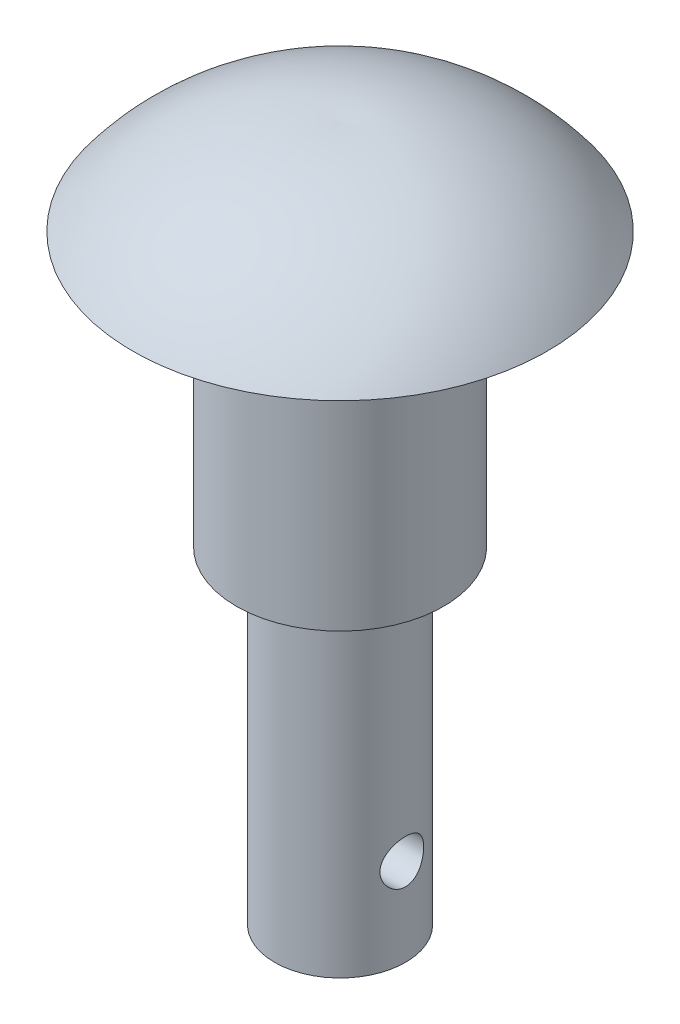
ISO-10303-21;
HEADER;
FILE_DESCRIPTION(('STEP AP214'),'2;1');
FILE_NAME('part.step','',(''),(''),'','','');
FILE_SCHEMA(('AUTOMOTIVE_DESIGN { 1 0 10303 214 1 1 1 1 }'));
ENDSEC;
DATA;
#1=APPLICATION_CONTEXT('core data for automotive mechanical design processes');
#2=APPLICATION_PROTOCOL_DEFINITION('international standard','automotive_design',2000,#1);
#3=PRODUCT_CONTEXT('',#1,'mechanical');
#4=PRODUCT('Part','Part','',(#3));
#5=PRODUCT_RELATED_PRODUCT_CATEGORY('part','',(#4));
#6=PRODUCT_DEFINITION_FORMATION('','',#4);
#7=PRODUCT_DEFINITION_CONTEXT('part definition',#1,'design');
#8=PRODUCT_DEFINITION('design','',#6,#7);
#9=PRODUCT_DEFINITION_SHAPE('','',#8);
#10=(LENGTH_UNIT() NAMED_UNIT(*) SI_UNIT(.MILLI.,.METRE.));
#11=(NAMED_UNIT(*) PLANE_ANGLE_UNIT() SI_UNIT($,.RADIAN.));
#12=(NAMED_UNIT(*) SI_UNIT($,.STERADIAN.) SOLID_ANGLE_UNIT());
#13=UNCERTAINTY_MEASURE_WITH_UNIT(LENGTH_MEASURE(1.E-05),#10,'distance_accuracy_value','');
#14=(GEOMETRIC_REPRESENTATION_CONTEXT(3) GLOBAL_UNCERTAINTY_ASSIGNED_CONTEXT((#13)) GLOBAL_UNIT_ASSIGNED_CONTEXT((#10,
#11,#12)) REPRESENTATION_CONTEXT('',''));
#15=CARTESIAN_POINT('',(0.,0.,0.));
#16=DIRECTION('',(0.,0.,1.));
#17=DIRECTION('',(1.,0.,0.));
#18=AXIS2_PLACEMENT_3D('',#15,#16,#17);
#19=CARTESIAN_POINT('',(0.,30.,0.));
#20=DIRECTION('',(0.,-1.,0.));
#21=DIRECTION('',(0.,0.,-1.));
#22=AXIS2_PLACEMENT_3D('',#19,#20,#21);
#23=CYLINDRICAL_SURFACE('',#22,6.);
#24=CARTESIAN_POINT('',(-5.65685424949238,8.,-2.));
#25=CARTESIAN_POINT('',(-5.65685389060868,8.10893634967214,-2.00000051589543));
#26=CARTESIAN_POINT('',(-5.66003538581715,8.21786959964719,-1.99106956737105));
#27=CARTESIAN_POINT('',(-5.67235148162509,8.4325088419885,-1.95570226337762));
#28=CARTESIAN_POINT('',(-5.68148706284377,8.53821429974494,-1.92926302433679));
#29=CARTESIAN_POINT('',(-5.70456407377583,8.74325378599457,-1.85991097136981));
#30=CARTESIAN_POINT('',(-5.71849607942643,8.84259985888543,-1.81703044280649));
#31=CARTESIAN_POINT('',(-5.74958244020649,9.03272009709592,-1.71612325688276));
#32=CARTESIAN_POINT('',(-5.76673750607224,9.12349236510726,-1.65809325772037));
#33=CARTESIAN_POINT('',(-5.80308978814946,9.29743992467663,-1.52610229288576));
#34=CARTESIAN_POINT('',(-5.82233789689288,9.38023085734346,-1.45164868275584));
#35=CARTESIAN_POINT('',(-5.86027729602006,9.53241360244928,-1.28997533442879));
#36=CARTESIAN_POINT('',(-5.87896849657923,9.60180326316474,-1.20275355010475));
#37=CARTESIAN_POINT('',(-5.91427733843598,9.72695779465919,-1.01520901593002));
#38=CARTESIAN_POINT('',(-5.93082815403211,9.78231994123592,-0.914603822449051));
#39=CARTESIAN_POINT('',(-5.95939173541966,9.87518317025502,-0.704862445974949));
#40=CARTESIAN_POINT('',(-5.97140572406004,9.91268906635381,-0.595728571374426));
#41=CARTESIAN_POINT('',(-5.98918150863813,9.96747170926479,-0.376057634866991));
#42=CARTESIAN_POINT('',(-5.99514629555118,9.98540689251401,-0.265701509705939));
#43=CARTESIAN_POINT('',(-6.00087216436495,10.0026325867213,-0.0433957496481808));
#44=CARTESIAN_POINT('',(-6.00063484525791,10.0019279033048,0.068553467087791));
#45=CARTESIAN_POINT('',(-5.99412079237462,9.98231149086794,0.286207030387628));
#46=CARTESIAN_POINT('',(-5.98808129510235,9.96411494305102,0.391984097183312));
#47=CARTESIAN_POINT('',(-5.97093934679463,9.91121403803906,0.598886877644342));
#48=CARTESIAN_POINT('',(-5.95983655262363,9.87650856204035,0.70001227555843));
#49=CARTESIAN_POINT('',(-5.93351340586448,9.79115736538788,0.896304949683944));
#50=CARTESIAN_POINT('',(-5.91824085048031,9.74030812290698,0.991376441937689));
#51=CARTESIAN_POINT('',(-5.88516786077838,9.62428058910269,1.17184865105464));
#52=CARTESIAN_POINT('',(-5.86736672402933,9.55909831334474,1.25724666877068));
#53=CARTESIAN_POINT('',(-5.83012383699793,9.4126512130806,1.42020173310261));
#54=CARTESIAN_POINT('',(-5.81064430337755,9.33077368431704,1.49720031413054));
#55=CARTESIAN_POINT('',(-5.77294670497801,9.15510254854676,1.63655451919635));
#56=CARTESIAN_POINT('',(-5.75472883491231,9.06130710854391,1.69890788656309));
#57=CARTESIAN_POINT('',(-5.72141050242224,8.86269274879312,1.80797491007149));
#58=CARTESIAN_POINT('',(-5.70635818569496,8.75773573736445,1.85445292724268));
#59=CARTESIAN_POINT('',(-5.68163301648769,8.54085721157116,1.92888638653867));
#60=CARTESIAN_POINT('',(-5.67195790974185,8.42893863758751,1.95684959149499));
#61=CARTESIAN_POINT('',(-5.6595927263117,8.20672328917685,1.99232256419504));
#62=CARTESIAN_POINT('',(-5.65660720637512,8.09658115050269,2.00069819101527));
#63=CARTESIAN_POINT('',(-5.65713344118368,7.87644770177179,1.99921087781944));
#64=CARTESIAN_POINT('',(-5.66064401583629,7.76645636795203,1.98935125045353));
#65=CARTESIAN_POINT('',(-5.67347236180599,7.55368606857618,1.95245130310462));
#66=CARTESIAN_POINT('',(-5.6825865088168,7.45078913969832,1.92601278796137));
#67=CARTESIAN_POINT('',(-5.70537107342046,7.25091278752163,1.85742772512094));
#68=CARTESIAN_POINT('',(-5.71904229869679,7.15393441681844,1.81527839272685));
#69=CARTESIAN_POINT('',(-5.74993755191574,6.96523915830601,1.71494868147787));
#70=CARTESIAN_POINT('',(-5.76726051331256,6.8737867147164,1.65630223671699));
#71=CARTESIAN_POINT('',(-5.8033153746193,6.70170789523256,1.52517126111512));
#72=CARTESIAN_POINT('',(-5.82204768887588,6.62108472267756,1.45268265099756));
#73=CARTESIAN_POINT('',(-5.85990077275698,6.46894403181872,1.29178341180065));
#74=CARTESIAN_POINT('',(-5.87899687155793,6.3980512199623,1.20277454109331));
#75=CARTESIAN_POINT('',(-5.91453703226217,6.27216771530392,1.01365458280052));
#76=CARTESIAN_POINT('',(-5.93098118835389,6.21717645767515,0.913543889729106));
#77=CARTESIAN_POINT('',(-5.95928811621206,6.12515979027657,0.705559724864593));
#78=CARTESIAN_POINT('',(-5.97118060009062,6.08801744570387,0.597742246642395));
#79=CARTESIAN_POINT('',(-5.98917221675549,6.03254451587979,0.376916931692035));
#80=CARTESIAN_POINT('',(-5.99527344068037,6.014207140239,0.263910983907781));
#81=CARTESIAN_POINT('',(-6.00083726472513,5.99747584478872,0.0416306717200839));
#82=CARTESIAN_POINT('',(-6.00059840178878,5.99818509213525,-0.0675694478400351));
#83=CARTESIAN_POINT('',(-5.99424393038796,6.01731461629282,-0.284222290000346));
#84=CARTESIAN_POINT('',(-5.98812879867151,6.03573345630554,-0.391675153638112));
#85=CARTESIAN_POINT('',(-5.97081829908824,6.08916446915192,-0.600084238864116));
#86=CARTESIAN_POINT('',(-5.95970516722297,6.12390843070586,-0.701116541825576));
#87=CARTESIAN_POINT('',(-5.9335432140899,6.20875506219431,-0.895956701879589));
#88=CARTESIAN_POINT('',(-5.91849368096033,6.25886051039403,-0.989763248284863));
#89=CARTESIAN_POINT('',(-5.88531737655762,6.37513902420401,-1.17126803261757));
#90=CARTESIAN_POINT('',(-5.86709744983853,6.44183737076328,-1.25861250311521));
#91=CARTESIAN_POINT('',(-5.82985977583759,6.58851478231239,-1.42116205254485));
#92=CARTESIAN_POINT('',(-5.81084177546194,6.66849808452545,-1.49636324324918));
#93=CARTESIAN_POINT('',(-5.77326559651196,6.8432187111739,-1.63548361766623));
#94=CARTESIAN_POINT('',(-5.75475455977261,6.93841102195328,-1.6988459319958));
#95=CARTESIAN_POINT('',(-5.7212038664603,7.13866885380556,-1.80862868660223));
#96=CARTESIAN_POINT('',(-5.70616330322498,7.24373178605933,-1.85505355363895));
#97=CARTESIAN_POINT('',(-5.68202668413029,7.45592364803126,-1.92768765640833));
#98=CARTESIAN_POINT('',(-5.67269265714364,7.56274452705073,-1.95471581829904));
#99=CARTESIAN_POINT('',(-5.66010767079036,7.7797121009334,-1.99086864029853));
#100=CARTESIAN_POINT('',(-5.65685461234922,7.88985763482142,-1.99999947839318));
#101=CARTESIAN_POINT('',(-5.65685424949238,8.,-2.));
#102=B_SPLINE_CURVE_WITH_KNOTS('',3,(#24,#25,#26,#27,#28,#29,#30,#31,#32,#33,#34,#35,#36,#37,
#38,#39,#40,#41,#42,#43,#44,#45,#46,#47,#48,#49,#50,#51,#52,#53,#54,#55,#56,#57,#58,#59,#60,#61,
#62,#63,#64,#65,#66,#67,#68,#69,#70,#71,#72,#73,#74,#75,#76,#77,#78,#79,#80,#81,#82,#83,#84,#85,
#86,#87,#88,#89,#90,#91,#92,#93,#94,#95,#96,#97,#98,#99,#100,#101),.UNSPECIFIED.,.T.,.F.,(4,2,2,
2,2,2,2,2,2,2,2,2,2,2,2,2,2,2,2,2,2,2,2,2,2,2,2,2,2,2,2,2,2,2,2,2,2,2,4),(0.,0.326401169598711,
0.652856110030327,0.978673255001655,1.30456233237088,1.64202674855136,1.97954530343976,
2.32587012287314,2.67210152773578,3.00628637529868,3.34038506604654,3.66138009651138,
3.98239688378473,4.3076330972067,4.63295983748044,4.97360348727835,5.31429959224212,
5.65985279686111,6.00526102713231,6.33508582728879,6.66485071674467,6.98328791537552,
7.30178158293891,7.6303771547143,7.95906971324255,8.30357616342185,8.64807037515064,
8.99027582381703,9.33235766008313,9.65836169355271,9.98433928019562,10.3051391208086,
10.6259970152648,10.9587103904127,11.2915300886526,11.6373780547229,11.9831355653373,
12.3132642432538,12.6432789438093),.UNSPECIFIED.);
#103=CARTESIAN_POINT('',(-5.65685424949238,8.,-2.));
#104=VERTEX_POINT('',#103);
#105=EDGE_CURVE('E47',#104,#104,#102,.T.);
#106=ORIENTED_EDGE('',*,*,#105,.T.);
#107=EDGE_LOOP('',(#106));
#108=FACE_BOUND('',#107,.T.);
#109=CARTESIAN_POINT('',(5.65685424949238,8.,-2.));
#110=CARTESIAN_POINT('',(5.65685389060868,7.89106365032786,-2.00000051589543));
#111=CARTESIAN_POINT('',(5.66003538581715,7.78213040035282,-1.99106956737105));
#112=CARTESIAN_POINT('',(5.67235148162509,7.5674911580115,-1.95570226337762));
#113=CARTESIAN_POINT('',(5.68148706284377,7.46178570025506,-1.92926302433679));
#114=CARTESIAN_POINT('',(5.70456407377583,7.25674621400542,-1.85991097136981));
#115=CARTESIAN_POINT('',(5.71849607942643,7.15740014111457,-1.81703044280649));
#116=CARTESIAN_POINT('',(5.74958244020649,6.96727990290408,-1.71612325688276));
#117=CARTESIAN_POINT('',(5.76673750607224,6.87650763489274,-1.65809325772037));
#118=CARTESIAN_POINT('',(5.80308978814946,6.70256007532337,-1.52610229288576));
#119=CARTESIAN_POINT('',(5.82233789689288,6.61976914265655,-1.45164868275584));
#120=CARTESIAN_POINT('',(5.86027729602006,6.46758639755072,-1.28997533442879));
#121=CARTESIAN_POINT('',(5.87896849657923,6.39819673683526,-1.20275355010475));
#122=CARTESIAN_POINT('',(5.91427733843598,6.27304220534081,-1.01520901593002));
#123=CARTESIAN_POINT('',(5.93082815403211,6.21768005876408,-0.914603822449051));
#124=CARTESIAN_POINT('',(5.95939173541966,6.12481682974498,-0.704862445974948));
#125=CARTESIAN_POINT('',(5.97140572406004,6.08731093364619,-0.595728571374425));
#126=CARTESIAN_POINT('',(5.98918150863813,6.03252829073521,-0.37605763486699));
#127=CARTESIAN_POINT('',(5.99514629555118,6.01459310748599,-0.265701509705938));
#128=CARTESIAN_POINT('',(6.00087216436495,5.99736741327868,-0.0433957496481801));
#129=CARTESIAN_POINT('',(6.00063484525791,5.99807209669518,0.0685534670877917));
#130=CARTESIAN_POINT('',(5.99412079237462,6.01768850913206,0.286207030387628));
#131=CARTESIAN_POINT('',(5.98808129510235,6.03588505694898,0.391984097183312));
#132=CARTESIAN_POINT('',(5.97093934679463,6.08878596196095,0.598886877644342));
#133=CARTESIAN_POINT('',(5.95983655262363,6.12349143795965,0.70001227555843));
#134=CARTESIAN_POINT('',(5.93351340586448,6.20884263461212,0.896304949683944));
#135=CARTESIAN_POINT('',(5.91824085048031,6.25969187709302,0.991376441937689));
#136=CARTESIAN_POINT('',(5.88516786077838,6.37571941089731,1.17184865105464));
#137=CARTESIAN_POINT('',(5.86736672402933,6.44090168665526,1.25724666877068));
#138=CARTESIAN_POINT('',(5.83012383699793,6.5873487869194,1.42020173310261));
#139=CARTESIAN_POINT('',(5.81064430337755,6.66922631568296,1.49720031413054));
#140=CARTESIAN_POINT('',(5.77294670497801,6.84489745145324,1.63655451919635));
#141=CARTESIAN_POINT('',(5.75472883491231,6.93869289145609,1.69890788656309));
#142=CARTESIAN_POINT('',(5.72141050242224,7.13730725120688,1.80797491007149));
#143=CARTESIAN_POINT('',(5.70635818569496,7.24226426263555,1.85445292724268));
#144=CARTESIAN_POINT('',(5.68163301648769,7.45914278842883,1.92888638653867));
#145=CARTESIAN_POINT('',(5.67195790974185,7.57106136241249,1.95684959149499));
#146=CARTESIAN_POINT('',(5.6595927263117,7.79327671082315,1.99232256419504));
#147=CARTESIAN_POINT('',(5.65660720637512,7.90341884949731,2.00069819101527));
#148=CARTESIAN_POINT('',(5.65713344118368,8.12355229822821,1.99921087781944));
#149=CARTESIAN_POINT('',(5.66064401583629,8.23354363204798,1.98935125045353));
#150=CARTESIAN_POINT('',(5.67347236180599,8.44631393142382,1.95245130310462));
#151=CARTESIAN_POINT('',(5.6825865088168,8.54921086030168,1.92601278796137));
#152=CARTESIAN_POINT('',(5.70537107342046,8.74908721247837,1.85742772512093));
#153=CARTESIAN_POINT('',(5.71904229869679,8.84606558318156,1.81527839272684));
#154=CARTESIAN_POINT('',(5.74993755191574,9.034760841694,1.71494868147787));
#155=CARTESIAN_POINT('',(5.76726051331256,9.1262132852836,1.65630223671699));
#156=CARTESIAN_POINT('',(5.8033153746193,9.29829210476744,1.52517126111512));
#157=CARTESIAN_POINT('',(5.82204768887588,9.37891527732244,1.45268265099756));
#158=CARTESIAN_POINT('',(5.85990077275698,9.53105596818128,1.29178341180065));
#159=CARTESIAN_POINT('',(5.87899687155793,9.6019487800377,1.20277454109331));
#160=CARTESIAN_POINT('',(5.91453703226217,9.72783228469608,1.01365458280051));
#161=CARTESIAN_POINT('',(5.93098118835389,9.78282354232485,0.913543889729105));
#162=CARTESIAN_POINT('',(5.95928811621206,9.87484020972343,0.705559724864591));
#163=CARTESIAN_POINT('',(5.97118060009062,9.91198255429613,0.597742246642394));
#164=CARTESIAN_POINT('',(5.98917221675549,9.96745548412021,0.376916931692034));
#165=CARTESIAN_POINT('',(5.99527344068037,9.98579285976101,0.26391098390778));
#166=CARTESIAN_POINT('',(6.00083726472513,10.0025241552113,0.0416306717200829));
#167=CARTESIAN_POINT('',(6.00059840178878,10.0018149078648,-0.067569447840036));
#168=CARTESIAN_POINT('',(5.99424393038796,9.98268538370718,-0.284222290000347));
#169=CARTESIAN_POINT('',(5.98812879867151,9.96426654369446,-0.391675153638113));
#170=CARTESIAN_POINT('',(5.97081829908824,9.91083553084808,-0.600084238864117));
#171=CARTESIAN_POINT('',(5.95970516722297,9.87609156929413,-0.701116541825577));
#172=CARTESIAN_POINT('',(5.9335432140899,9.79124493780569,-0.89595670187959));
#173=CARTESIAN_POINT('',(5.91849368096033,9.74113948960598,-0.989763248284864));
#174=CARTESIAN_POINT('',(5.88531737655762,9.62486097579599,-1.17126803261757));
#175=CARTESIAN_POINT('',(5.86709744983853,9.55816262923672,-1.25861250311521));
#176=CARTESIAN_POINT('',(5.82985977583759,9.41148521768761,-1.42116205254485));
#177=CARTESIAN_POINT('',(5.81084177546194,9.33150191547455,-1.49636324324918));
#178=CARTESIAN_POINT('',(5.77326559651196,9.1567812888261,-1.63548361766623));
#179=CARTESIAN_POINT('',(5.75475455977261,9.06158897804672,-1.6988459319958));
#180=CARTESIAN_POINT('',(5.7212038664603,8.86133114619444,-1.80862868660223));
#181=CARTESIAN_POINT('',(5.70616330322498,8.75626821394067,-1.85505355363895));
#182=CARTESIAN_POINT('',(5.68202668413029,8.54407635196874,-1.92768765640833));
#183=CARTESIAN_POINT('',(5.67269265714364,8.43725547294927,-1.95471581829904));
#184=CARTESIAN_POINT('',(5.66010767079036,8.2202878990666,-1.99086864029853));
#185=CARTESIAN_POINT('',(5.65685461234922,8.11014236517858,-1.99999947839318));
#186=CARTESIAN_POINT('',(5.65685424949238,8.,-2.));
#187=B_SPLINE_CURVE_WITH_KNOTS('',3,(#109,#110,#111,#112,#113,#114,#115,#116,#117,#118,#119,
#120,#121,#122,#123,#124,#125,#126,#127,#128,#129,#130,#131,#132,#133,#134,#135,#136,#137,#138,
#139,#140,#141,#142,#143,#144,#145,#146,#147,#148,#149,#150,#151,#152,#153,#154,#155,#156,#157,
#158,#159,#160,#161,#162,#163,#164,#165,#166,#167,#168,#169,#170,#171,#172,#173,#174,#175,#176,
#177,#178,#179,#180,#181,#182,#183,#184,#185,#186),.UNSPECIFIED.,.T.,.F.,(4,2,2,2,2,2,2,2,2,2,2,
2,2,2,2,2,2,2,2,2,2,2,2,2,2,2,2,2,2,2,2,2,2,2,2,2,2,2,4),(0.,0.326401169598712,
0.652856110030327,0.978673255001655,1.30456233237088,1.64202674855136,1.97954530343976,
2.32587012287314,2.67210152773578,3.00628637529868,3.34038506604655,3.66138009651138,
3.98239688378473,4.3076330972067,4.63295983748044,4.97360348727835,5.31429959224212,
5.65985279686111,6.00526102713231,6.33508582728879,6.66485071674468,6.98328791537552,
7.30178158293892,7.6303771547143,7.95906971324254,8.30357616342185,8.64807037515065,
8.99027582381703,9.33235766008313,9.65836169355271,9.98433928019562,10.3051391208086,
10.6259970152649,10.9587103904127,11.2915300886526,11.6373780547229,11.9831355653373,
12.3132642432538,12.6432789438093),.UNSPECIFIED.);
#188=CARTESIAN_POINT('',(5.65685424949238,8.,-2.));
#189=VERTEX_POINT('',#188);
#190=EDGE_CURVE('E93',#189,#189,#187,.T.);
#191=ORIENTED_EDGE('',*,*,#190,.T.);
#192=EDGE_LOOP('',(#191));
#193=FACE_BOUND('',#192,.T.);
#194=CARTESIAN_POINT('',(0.,30.,0.));
#195=DIRECTION('',(0.,1.,0.));
#196=DIRECTION('',(0.,0.,1.));
#197=AXIS2_PLACEMENT_3D('',#194,#195,#196);
#198=CIRCLE('',#197,6.);
#199=CARTESIAN_POINT('',(0.,30.,6.));
#200=VERTEX_POINT('',#199);
#201=EDGE_CURVE('E11',#200,#200,#198,.T.);
#202=ORIENTED_EDGE('',*,*,#201,.F.);
#203=EDGE_LOOP('',(#202));
#204=FACE_BOUND('',#203,.T.);
#205=CARTESIAN_POINT('',(0.,0.,0.));
#206=DIRECTION('',(0.,1.,0.));
#207=DIRECTION('',(0.,0.,1.));
#208=AXIS2_PLACEMENT_3D('',#205,#206,#207);
#209=CIRCLE('',#208,6.);
#210=CARTESIAN_POINT('',(0.,0.,6.));
#211=VERTEX_POINT('',#210);
#212=EDGE_CURVE('E60',#211,#211,#209,.T.);
#213=ORIENTED_EDGE('',*,*,#212,.T.);
#214=EDGE_LOOP('',(#213));
#215=FACE_BOUND('',#214,.T.);
#216=ADVANCED_FACE('F44',(#108,#193,#204,#215),#23,.T.);
#217=CARTESIAN_POINT('',(0.,0.,0.));
#218=DIRECTION('',(0.,1.,0.));
#219=DIRECTION('',(0.,0.,1.));
#220=AXIS2_PLACEMENT_3D('',#217,#218,#219);
#221=PLANE('',#220);
#222=ORIENTED_EDGE('',*,*,#212,.F.);
#223=EDGE_LOOP('',(#222));
#224=FACE_BOUND('',#223,.T.);
#225=ADVANCED_FACE('F80',(#224),#221,.F.);
#226=CARTESIAN_POINT('',(0.,55.,0.));
#227=DIRECTION('',(0.,-1.,0.));
#228=DIRECTION('',(0.,0.,-1.));
#229=AXIS2_PLACEMENT_3D('',#226,#227,#228);
#230=CYLINDRICAL_SURFACE('',#229,9.5);
#231=CARTESIAN_POINT('',(0.,55.,0.));
#232=DIRECTION('',(0.,1.,0.));
#233=DIRECTION('',(0.,0.,1.));
#234=AXIS2_PLACEMENT_3D('',#231,#232,#233);
#235=CIRCLE('',#234,9.5);
#236=CARTESIAN_POINT('',(0.,55.,9.5));
#237=VERTEX_POINT('',#236);
#238=EDGE_CURVE('E96',#237,#237,#235,.T.);
#239=ORIENTED_EDGE('',*,*,#238,.F.);
#240=EDGE_LOOP('',(#239));
#241=FACE_BOUND('',#240,.T.);
#242=CARTESIAN_POINT('',(0.,30.,0.));
#243=DIRECTION('',(0.,1.,0.));
#244=DIRECTION('',(0.,0.,1.));
#245=AXIS2_PLACEMENT_3D('',#242,#243,#244);
#246=CIRCLE('',#245,9.5);
#247=CARTESIAN_POINT('',(0.,30.,9.5));
#248=VERTEX_POINT('',#247);
#249=EDGE_CURVE('E97',#248,#248,#246,.T.);
#250=ORIENTED_EDGE('',*,*,#249,.T.);
#251=EDGE_LOOP('',(#250));
#252=FACE_BOUND('',#251,.T.);
#253=ADVANCED_FACE('F85',(#241,#252),#230,.T.);
#254=CARTESIAN_POINT('',(0.,30.,0.));
#255=DIRECTION('',(0.,1.,0.));
#256=DIRECTION('',(0.,0.,1.));
#257=AXIS2_PLACEMENT_3D('',#254,#255,#256);
#258=PLANE('',#257);
#259=ORIENTED_EDGE('',*,*,#201,.T.);
#260=EDGE_LOOP('',(#259));
#261=FACE_BOUND('',#260,.T.);
#262=ORIENTED_EDGE('',*,*,#249,.F.);
#263=EDGE_LOOP('',(#262));
#264=FACE_BOUND('',#263,.T.);
#265=ADVANCED_FACE('F71',(#261,#264),#258,.F.);
#266=CARTESIAN_POINT('',(0.,55.,0.));
#267=DIRECTION('',(0.,1.,0.));
#268=DIRECTION('',(0.,0.,1.));
#269=AXIS2_PLACEMENT_3D('',#266,#267,#268);
#270=PLANE('',#269);
#271=ORIENTED_EDGE('',*,*,#238,.T.);
#272=EDGE_LOOP('',(#271));
#273=FACE_BOUND('',#272,.T.);
#274=CARTESIAN_POINT('',(0.,55.,0.));
#275=DIRECTION('',(0.,-1.,0.));
#276=DIRECTION('',(0.,0.,-1.));
#277=AXIS2_PLACEMENT_3D('',#274,#275,#276);
#278=CIRCLE('',#277,19.);
#279=CARTESIAN_POINT('',(0.,55.,-19.));
#280=VERTEX_POINT('',#279);
#281=EDGE_CURVE('E110',#280,#280,#278,.T.);
#282=ORIENTED_EDGE('',*,*,#281,.T.);
#283=EDGE_LOOP('',(#282));
#284=FACE_BOUND('',#283,.T.);
#285=ADVANCED_FACE('F63',(#273,#284),#270,.F.);
#286=CARTESIAN_POINT('',(0.,41.7804354672986,-1.41469040460922));
#287=DIRECTION('',(-1.,0.,0.));
#288=DIRECTION('',(0.,0.,-1.));
#289=AXIS2_PLACEMENT_3D('',#286,#287,#288);
#290=CIRCLE('',#289,22.);
#291=TRIMMED_CURVE('',#290,(PARAMETER_VALUE(-1.63514483520769)),
(PARAMETER_VALUE(1.63514483520769)),.T.,.PARAMETER.);
#292=CARTESIAN_POINT('',(0.,41.7804354672986,0.));
#293=DIRECTION('',(0.,-1.,0.));
#294=AXIS1_PLACEMENT('',#292,#293);
#295=SURFACE_OF_REVOLUTION('',#291,#294);
#296=ORIENTED_EDGE('',*,*,#281,.F.);
#297=EDGE_LOOP('',(#296));
#298=FACE_BOUND('',#297,.T.);
#299=CARTESIAN_POINT('',(0.,63.7349031460902,0.));
#300=VERTEX_POINT('',#299);
#301=VERTEX_LOOP('',#300);
#302=FACE_BOUND('',#301,.T.);
#303=ADVANCED_FACE('F61',(#298,#302),#295,.T.);
#304=CARTESIAN_POINT('',(-12.5,8.,0.));
#305=DIRECTION('',(1.,0.,0.));
#306=DIRECTION('',(0.,0.,-1.));
#307=AXIS2_PLACEMENT_3D('',#304,#305,#306);
#308=CYLINDRICAL_SURFACE('',#307,2.);
#309=ORIENTED_EDGE('',*,*,#190,.F.);
#310=EDGE_LOOP('',(#309));
#311=FACE_BOUND('',#310,.T.);
#312=ORIENTED_EDGE('',*,*,#105,.F.);
#313=EDGE_LOOP('',(#312));
#314=FACE_BOUND('',#313,.T.);
#315=ADVANCED_FACE('F62',(#311,#314),#308,.F.);
#316=CLOSED_SHELL('',(#216,#225,#253,#265,#285,#303,#315));
#317=MANIFOLD_SOLID_BREP('B2',#316);
#318=ADVANCED_BREP_SHAPE_REPRESENTATION('',(#18,#317),#14);
#319=SHAPE_DEFINITION_REPRESENTATION(#9,#318);
ENDSEC;
END-ISO-10303-21;
